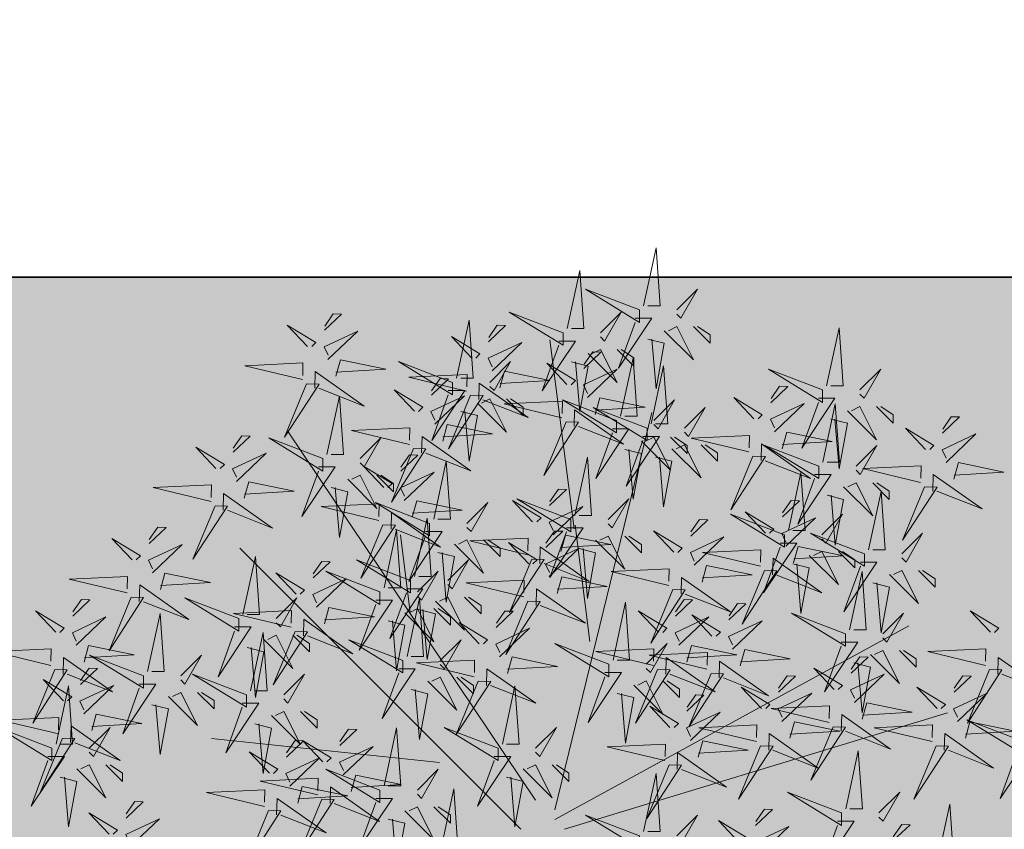
# Model space of a CAD drawing. Units: inches. Extents: x 1704 to 6393, y -157 to 1172.
# Tile 113 of 122: x 2688 to 2716, y 1018 to 1041. Entities that reach past the tile are written whole.
import ezdxf

# ---------------------------------------------------------------- set-up
doc = ezdxf.new("R2010")
doc.units = ezdxf.units.IN
doc.header["$MEASUREMENT"] = 0
for name, color, linetype, lineweight in [('A-ANNO-DIMS', 7, 'Continuous', 13), ('C-PROP', 7, 'Continuous', 35), ('L-shrub', 74, 'Continuous', 18)]:
    doc.layers.add(name, color=color, linetype=linetype, lineweight=lineweight)
doc.layers.add('L-HRDS-PATT', color=9, linetype='Continuous', lineweight=13, true_color=0xc5c1ba)
doc.styles.get("Standard").update_dxf_attribs({"font": 'arial.ttf'})
doc.dimstyles.get("Standard").update_dxf_attribs({"dimtxt": 6, "dimasz": 2, "dimexe": 0.18, "dimexo": 0.0625, "dimgap": 0.09, "dimtad": 0, "dimtih": 1, "dimtoh": 1, "dimdec": 1, "dimzin": 0, "dimdsep": 46, "dimlunit": 3, "dimtxsty": 'Standard', "dimblk": 'ARCHTICK', "dimcen": 0.09, "dimadec": 0, "dimazin": 0, "dimtfac": 1, "dimtdec": 1, "dimtofl": 0, "dimtmove": 0, "dimatfit": 3, "dimfxl": 1, "dimtolj": 1, "dimtzin": 0, "dimarcsym": 0})

# ---------------------------------------------------------------- blocks, each defined once
blk = doc.blocks.new('shrub3')
for p, q in [((-11.38, -5.19), (-224.23, -69.78)), ((12.87, -5.19), (169.14, -161.27)), ((-5.99, -10.57), (-202.68, -118.21)), ((-5.99, -15.96), (-59.88, -236.62)), ((4.78, -21.34), (142.19, -225.85)), ((58.17, -42.16), (184.8, -55.61)), ((-17.27, -174.02), (-25.36, -109.43)), ((74.33, -125.58), (79.72, -168.64)), ((-16.77, -172.03), (-3.3, -276.98))]:
    blk.add_line(p, q)
for points in [[(-163.04, -9.56), (-172.27, -9.56), (-153.8, 18.11), (-163.04, -7.25)], [(86.56, -10.73), (77.32, -8.43), (81.94, 16.94), (84.25, -10.73)], [(-218.53, 13.17), (-225.46, -19.11), (-227.77, 13.17), (-220.84, 13.17)], [(153.14, -15.45), (165.42, 14.26), (146.23, -15.28), (153.14, -15.45)], [(-119.49, 9.1), (-136.03, -6.65), (-117.36, 2.12), (-119.55, 6.79)], [(123.46, -21.81), (135.74, 7.91), (116.55, -21.63), (123.46, -21.81)], [(-193.91, 1.36), (-203.36, -7.64), (-198.75, -7.76), (-193.97, -0.95)], [(-108.14, 1.89), (-96.9, -9.94), (-112.81, -0.3), (-110.44, 1.95)], [(-73.76, -1.46), (-85.3, -12.99), (-76.07, 3.15), (-73.76, 0.84)], [(-52.98, -1.46), (-22.97, -12.99), (-52.98, 5.45), (-52.98, -1.46)], [(57.07, 4.7), (50.14, -27.58), (47.83, 4.7), (54.76, 4.7)], [(77.32, -15.34), (61.16, 0.8), (70.4, -17.65), (75.02, -15.34)], [(93.49, -22.26), (84.25, -22.26), (102.72, 5.41), (93.49, -19.96)], [(230.31, 4.87), (213.77, -10.89), (232.44, -2.12), (230.25, 2.56)], [(-55.29, -3.77), (-62.22, -36.05), (-64.53, -3.77), (-57.6, -3.77)], [(148.59, -13.03), (148.36, -22.26), (121.16, -3.11), (146.29, -12.97)], [(241.66, -2.35), (252.9, -14.18), (237, -4.54), (239.36, -2.29)], [(-186.12, -14.17), (-197.67, -25.7), (-188.43, -9.56), (-186.12, -11.86)], [(-165.34, -14.17), (-135.33, -25.7), (-165.34, -7.25), (-165.34, -14.17)], [(-117.59, -7.11), (-127.04, -16.11), (-122.43, -16.23), (-117.65, -9.42)], [(20.84, -34.02), (11.6, -31.72), (16.22, -6.36), (18.53, -34.02)], [(61.16, -17.65), (51.93, -8.43), (51.93, -13.04), (58.86, -17.65)], [(118.91, -19.38), (118.68, -28.61), (91.48, -9.46), (116.61, -19.33)], [(268.88, -34.02), (259.65, -31.72), (264.26, -6.36), (266.57, -34.02)], [(-69.46, -40.86), (-57.18, -11.15), (-76.37, -40.69), (-69.46, -40.86)], [(232.21, -11.35), (222.76, -20.35), (227.37, -20.46), (232.16, -13.66)], [(-217.86, -51.45), (-205.58, -21.74), (-224.77, -51.28), (-217.86, -51.45)], [(-167.65, -16.47), (-174.58, -48.76), (-176.89, -16.47), (-169.96, -16.47)], [(-120.34, -51.45), (-108.06, -21.74), (-127.25, -51.28), (-120.34, -51.45)], [(27.76, -45.55), (18.53, -45.55), (37, -17.88), (27.76, -43.25)], [(91.18, -26.87), (121.19, -38.4), (91.18, -19.96), (91.18, -26.87)], [(136.89, -19.67), (134.36, -28.84), (109.12, -23.59), (136.84, -21.97)], [(155.39, -17.82), (187.49, -25.55), (155.16, -27.05), (155.33, -20.13)], [(275.81, -45.55), (266.57, -45.55), (285.04, -17.88), (275.81, -43.25)], [(-262.68, -49.79), (-271.91, -49.79), (-253.44, -22.12), (-262.68, -47.48)], [(11.6, -38.64), (-4.56, -22.5), (4.68, -40.94), (9.3, -38.64)], [(70.4, -26.87), (58.86, -38.4), (68.09, -22.26), (70.4, -24.57)], [(107.21, -26.02), (104.68, -35.19), (79.44, -29.94), (107.16, -28.33)], [(125.71, -24.17), (157.81, -31.9), (125.48, -33.4), (125.65, -26.48)], [(259.65, -38.64), (243.49, -22.5), (252.72, -40.94), (257.34, -38.64)], [(267.62, -55.68), (279.9, -25.97), (260.71, -55.51), (267.62, -55.68)], [(-160.62, -62.04), (-148.34, -32.32), (-167.53, -61.86), (-160.62, -62.04)], [(-74.01, -38.44), (-74.24, -47.67), (-101.44, -28.52), (-76.31, -38.38)], [(-4.56, -40.94), (-13.79, -31.72), (-13.79, -36.33), (-6.86, -40.94)], [(88.87, -29.18), (81.94, -61.46), (79.63, -29.18), (86.56, -29.18)], [(141.27, -29.01), (124.73, -44.76), (143.4, -35.99), (141.21, -31.32)], [(243.49, -40.94), (234.25, -31.72), (234.25, -36.33), (241.18, -40.94)], [(111.59, -35.37), (95.05, -51.12), (113.72, -42.35), (111.53, -37.67)], [(152.62, -36.23), (163.86, -48.05), (147.96, -38.42), (150.32, -36.17)], [(160.76, -63.67), (151.53, -61.36), (156.14, -36), (158.45, -63.67)], [(-222.41, -49.03), (-222.64, -58.26), (-249.84, -39.1), (-224.72, -48.97)], [(-124.89, -49.03), (-125.12, -58.26), (-152.32, -39.1), (-127.2, -48.97)], [(-67.21, -43.23), (-35.11, -50.96), (-67.44, -52.46), (-67.27, -45.54)], [(25.46, -50.16), (55.47, -61.69), (25.46, -43.25), (25.46, -50.16)], [(122.94, -42.58), (134.18, -54.41), (118.28, -44.77), (120.64, -42.52)], [(263.07, -53.26), (262.84, -62.49), (235.64, -43.34), (260.77, -53.2)], [(273.5, -50.16), (303.51, -61.69), (273.5, -43.25), (273.5, -50.16)], [(-264.99, -54.4), (-234.97, -65.93), (-264.99, -47.48), (-264.99, -54.4)], [(-85.71, -45.07), (-88.24, -54.25), (-113.48, -49), (-85.77, -47.38)], [(4.68, -50.16), (-6.86, -61.69), (2.37, -45.55), (4.68, -47.86)], [(143.17, -45.23), (133.72, -54.23), (138.33, -54.34), (143.12, -47.53)], [(167.69, -75.2), (158.45, -75.2), (176.92, -47.53), (167.69, -72.89)], [(218, -74.25), (208.77, -71.95), (213.38, -46.59), (215.69, -74.25)], [(252.72, -50.16), (241.18, -61.69), (250.41, -45.55), (252.72, -47.86)], [(-215.61, -53.82), (-183.51, -61.55), (-215.84, -63.05), (-215.67, -56.12)], [(-165.17, -59.61), (-165.4, -68.85), (-192.6, -49.69), (-167.48, -59.56)], [(-118.09, -53.82), (-85.99, -61.55), (-118.32, -63.05), (-118.15, -56.12)], [(-81.33, -54.42), (-97.87, -70.17), (-79.2, -61.4), (-81.39, -56.73)], [(-40.64, -80.61), (-49.88, -78.3), (-45.26, -52.94), (-42.95, -80.61)], [(23.15, -52.47), (16.22, -84.75), (13.91, -52.47), (20.84, -52.47)], [(113.49, -51.58), (104.04, -60.58), (108.65, -60.69), (113.43, -53.89)], [(151.53, -68.28), (135.37, -52.14), (144.6, -70.59), (149.22, -68.28)], [(271.19, -52.47), (264.26, -84.75), (261.95, -52.47), (268.88, -52.47)], [(-234.11, -55.66), (-236.65, -64.84), (-261.89, -59.59), (-234.17, -57.97)], [(-136.59, -55.66), (-139.12, -64.84), (-164.36, -59.59), (-136.65, -57.97)], [(36.54, -87.45), (48.82, -57.73), (29.63, -87.27), (36.54, -87.45)], [(73.84, -82.72), (64.6, -80.42), (69.22, -55.06), (71.53, -82.72)], [(224.93, -85.78), (215.69, -85.78), (234.16, -58.11), (224.93, -83.48)], [(251.37, -59.9), (248.84, -69.07), (223.6, -63.82), (251.32, -62.2)], [(269.87, -58.05), (301.97, -65.78), (269.64, -67.28), (269.81, -60.36)], [(-247.54, -93.8), (-235.26, -64.08), (-254.45, -93.62), (-247.54, -93.8)], [(-229.73, -65.01), (-246.27, -80.76), (-227.6, -71.99), (-229.79, -67.32)], [(-158.37, -64.4), (-126.27, -72.13), (-158.6, -73.63), (-158.43, -66.71)], [(-132.21, -65.01), (-148.75, -80.76), (-130.08, -71.99), (-132.27, -67.32)], [(-92.78, -91.68), (-80.5, -61.97), (-99.69, -91.51), (-92.78, -91.68)], [(-69.98, -61.63), (-58.74, -73.46), (-74.65, -63.83), (-72.28, -61.58)], [(-63.1, -93.8), (-50.82, -64.08), (-70.01, -93.62), (-63.1, -93.8)], [(-33.72, -92.14), (-42.95, -92.14), (-24.48, -64.47), (-33.72, -89.83)], [(135.37, -70.59), (126.13, -61.36), (126.13, -65.97), (133.06, -70.59)], [(208.77, -78.87), (192.61, -62.73), (201.84, -81.17), (206.46, -78.87)], [(271.86, -93.8), (284.14, -64.08), (264.95, -93.62), (271.86, -93.8)], [(-176.87, -66.25), (-179.4, -75.42), (-204.64, -70.17), (-176.93, -68.56)], [(-172.08, -97.55), (-181.32, -95.24), (-176.7, -69.88), (-174.39, -97.55)], [(-79.43, -70.63), (-88.88, -79.64), (-84.27, -79.75), (-79.49, -72.94)], [(-49.88, -85.22), (-66.04, -69.08), (-56.8, -87.52), (-52.18, -85.22)], [(80.77, -94.25), (71.53, -94.25), (90, -66.58), (80.77, -91.95)], [(255.75, -69.24), (239.21, -85), (257.88, -76.23), (255.7, -71.55)], [(-218.38, -72.22), (-207.14, -84.05), (-223.05, -74.41), (-220.68, -72.16)], [(-172.49, -75.6), (-189.03, -91.35), (-170.36, -82.58), (-172.55, -77.9)], [(-120.86, -72.22), (-109.62, -84.05), (-125.53, -74.41), (-123.16, -72.16)], [(31.99, -85.02), (31.76, -94.25), (4.56, -75.1), (29.69, -84.96)], [(64.6, -87.34), (48.44, -71.2), (57.68, -89.64), (62.3, -87.34)], [(144.6, -79.81), (133.06, -91.34), (142.29, -75.2), (144.6, -77.5)], [(165.38, -79.81), (195.39, -91.34), (165.38, -72.89), (165.38, -79.81)], [(192.61, -81.17), (183.37, -71.95), (183.37, -76.56), (190.3, -81.17)], [(267.1, -76.46), (278.34, -88.28), (262.44, -78.65), (264.8, -76.4)], [(-252.09, -91.37), (-252.32, -100.61), (-279.52, -81.45), (-254.4, -91.32)], [(-227.83, -81.22), (-237.28, -90.22), (-232.67, -90.34), (-227.89, -83.53)], [(-165.16, -109.08), (-174.39, -109.08), (-155.92, -81.41), (-165.16, -106.77)], [(-130.31, -81.22), (-139.76, -90.22), (-135.15, -90.34), (-130.37, -83.53)], [(-97.33, -89.26), (-97.56, -98.49), (-124.76, -79.33), (-99.63, -89.2)], [(-67.65, -91.37), (-67.88, -100.61), (-95.08, -81.45), (-69.95, -91.32)], [(-66.04, -87.52), (-75.27, -78.3), (-75.27, -82.91), (-68.34, -87.52)], [(48.44, -89.64), (39.21, -80.42), (39.21, -85.03), (46.14, -89.64)], [(165, -106.02), (155.77, -103.71), (160.38, -78.35), (162.69, -106.02)], [(267.31, -91.37), (267.08, -100.61), (239.88, -81.45), (265.01, -91.32)], [(-181.32, -102.16), (-197.48, -86.02), (-188.24, -104.46), (-183.63, -102.16)], [(-161.14, -82.81), (-149.9, -94.64), (-165.81, -85), (-163.44, -82.75)], [(138.3, -114.97), (150.58, -85.26), (131.39, -114.8), (138.3, -114.97)], [(163.07, -82.11), (156.14, -114.39), (153.83, -82.11), (160.76, -82.11)], [(201.84, -90.4), (190.3, -101.92), (199.53, -85.78), (201.84, -88.09)], [(222.62, -90.4), (252.63, -101.92), (222.62, -83.48), (222.62, -90.4)], [(257.65, -85.46), (248.2, -94.46), (252.81, -94.57), (257.6, -87.76)], [(-170.59, -91.81), (-180.04, -100.81), (-175.43, -100.93), (-170.65, -94.12)], [(-56.8, -96.75), (-68.34, -108.28), (-59.11, -92.14), (-56.8, -94.44)], [(-36.02, -96.75), (-6.01, -108.28), (-36.02, -89.83), (-36.02, -96.75)], [(20.29, -91.66), (17.76, -100.83), (-7.48, -95.58), (20.23, -93.97)], [(38.79, -89.81), (70.89, -97.54), (38.56, -99.04), (38.73, -92.12)], [(78.46, -98.86), (108.47, -110.39), (78.46, -91.95), (78.46, -98.86)], [(171.93, -117.54), (162.69, -117.54), (181.16, -89.88), (171.93, -115.24)], [(220.31, -92.7), (213.38, -124.98), (211.07, -92.7), (218, -92.7)], [(-245.29, -96.16), (-213.19, -103.89), (-245.52, -105.4), (-245.35, -98.47)], [(-197.48, -104.46), (-206.71, -95.24), (-206.71, -99.85), (-199.79, -104.46)], [(-109.03, -95.89), (-111.56, -105.07), (-136.8, -99.82), (-109.09, -98.2)], [(-79.35, -98.01), (-81.88, -107.18), (-107.12, -101.93), (-79.41, -100.32)], [(-90.53, -94.05), (-58.43, -101.78), (-90.76, -103.28), (-90.59, -96.35)], [(-60.85, -96.16), (-28.75, -103.89), (-61.08, -105.4), (-60.91, -98.47)], [(57.68, -98.86), (46.14, -110.39), (55.37, -94.25), (57.68, -96.56)], [(86.56, -120.84), (77.32, -118.53), (81.94, -93.17), (84.25, -120.84)], [(155.77, -110.63), (139.61, -94.49), (148.84, -112.93), (153.46, -110.63)], [(255.61, -98.01), (253.08, -107.18), (227.84, -101.93), (255.56, -100.32)], [(274.11, -96.16), (306.21, -103.89), (273.88, -105.4), (274.05, -98.47)], [(-38.33, -99.05), (-45.26, -131.33), (-47.57, -99.05), (-40.64, -99.05)], [(8.98, -131.91), (21.26, -102.2), (2.07, -131.74), (8.98, -131.91)], [(24.67, -101), (8.13, -116.76), (26.8, -107.99), (24.61, -103.31)], [(69.6, -127.19), (60.36, -124.88), (64.98, -99.52), (67.29, -127.19)], [(76.15, -101.17), (69.22, -133.45), (66.91, -101.17), (73.84, -101.17)], [(133.75, -112.55), (133.52, -121.78), (106.32, -102.62), (131.45, -112.49)], [(139.61, -112.93), (130.37, -103.71), (130.37, -108.32), (137.3, -112.93)], [(-188.24, -113.69), (-199.79, -125.22), (-190.55, -109.08), (-188.24, -111.38)], [(-167.46, -113.69), (-137.45, -125.22), (-167.46, -106.77), (-167.46, -113.69)], [(-104.65, -105.24), (-121.19, -120.99), (-102.52, -112.22), (-104.71, -107.55)], [(-74.97, -107.36), (-91.51, -123.11), (-72.84, -114.34), (-75.03, -109.66)], [(-71.58, -138.26), (-59.3, -108.55), (-78.49, -138.09), (-71.58, -138.26)], [(36.02, -108.22), (47.26, -120.04), (31.36, -110.41), (33.72, -108.16)], [(77.32, -125.45), (61.16, -109.31), (70.4, -127.75), (75.02, -125.45)], [(93.49, -132.37), (84.25, -132.37), (102.72, -104.7), (93.49, -130.06)], [(229.46, -134.03), (241.74, -104.31), (222.55, -133.86), (229.46, -134.03)], [(259.99, -107.36), (243.45, -123.11), (262.12, -114.34), (259.94, -109.66)], [(-248.06, -114.57), (-236.82, -126.4), (-252.73, -116.76), (-250.36, -114.51)], [(-182.68, -142.01), (-191.92, -139.71), (-187.3, -114.34), (-184.99, -142.01)], [(-93.3, -112.45), (-82.06, -124.28), (-97.97, -114.64), (-95.6, -112.39)], [(-63.62, -114.57), (-52.38, -126.4), (-68.29, -116.76), (-65.92, -114.51)], [(76.53, -138.72), (67.29, -138.72), (85.76, -111.05), (76.53, -136.41)], [(271.34, -114.57), (282.58, -126.4), (266.68, -116.76), (269.04, -114.51)], [(-169.77, -115.99), (-176.7, -148.27), (-179.01, -115.99), (-172.08, -115.99)], [(-122.46, -148.85), (-110.18, -119.14), (-129.37, -148.68), (-122.46, -148.85)], [(4.43, -129.49), (4.2, -138.72), (-23, -119.56), (2.13, -129.43)], [(26.57, -117.22), (17.12, -126.22), (21.73, -126.33), (26.51, -119.53)], [(60.36, -131.8), (44.2, -115.66), (53.44, -134.11), (58.06, -131.8)], [(61.16, -127.75), (51.93, -118.53), (51.93, -123.14), (58.86, -127.75)], [(122.05, -119.18), (119.52, -128.36), (94.28, -123.11), (122, -121.49)], [(148.84, -122.16), (137.3, -133.69), (146.53, -117.54), (148.84, -119.85)], [(140.55, -117.34), (172.65, -125.07), (140.32, -126.57), (140.49, -119.65)], [(169.62, -122.16), (199.63, -133.69), (169.62, -115.24), (169.62, -122.16)], [(-138.16, -152.6), (-147.4, -150.29), (-142.78, -124.93), (-140.47, -152.6)], [(-102.75, -121.45), (-112.2, -130.45), (-107.59, -130.57), (-102.81, -123.76)], [(-73.07, -123.57), (-82.52, -132.57), (-77.91, -132.69), (-73.13, -125.88)], [(6.86, -155.2), (19.14, -125.49), (-0.05, -155.03), (6.86, -155.2)], [(44.2, -134.11), (34.97, -124.88), (34.97, -129.5), (41.9, -134.11)], [(167.31, -124.46), (160.38, -156.74), (158.07, -124.46), (165, -124.46)], [(224.91, -131.61), (224.68, -140.84), (197.48, -121.68), (222.61, -131.55)], [(261.89, -123.57), (252.44, -132.57), (257.05, -132.69), (261.84, -125.88)], [(-191.92, -146.62), (-208.08, -130.48), (-198.84, -148.93), (-194.23, -146.62)], [(-175.76, -153.54), (-184.99, -153.54), (-166.52, -125.87), (-175.76, -151.23)], [(-76.13, -135.84), (-76.36, -145.07), (-103.56, -125.92), (-78.43, -135.78)], [(59, -158.95), (49.76, -156.64), (54.38, -131.28), (56.69, -158.95)], [(91.18, -136.98), (121.19, -148.51), (91.18, -130.06), (91.18, -136.98)], [(126.43, -128.53), (109.89, -144.28), (128.56, -135.51), (126.37, -130.84)], [(-127.01, -146.43), (-127.24, -155.66), (-154.44, -136.5), (-129.32, -146.37)], [(-131.24, -164.13), (-140.47, -164.13), (-122, -136.46), (-131.24, -161.82)], [(-7.27, -136.12), (-9.8, -145.3), (-35.04, -140.05), (-7.33, -138.43)], [(-19.44, -161.07), (-28.68, -158.76), (-24.06, -133.4), (-21.75, -161.07)], [(11.23, -134.28), (43.33, -142.01), (11, -143.51), (11.17, -136.58)], [(70.4, -136.98), (58.86, -148.51), (68.09, -132.37), (70.4, -134.67)], [(74.22, -143.33), (104.23, -154.86), (74.22, -136.41), (74.22, -143.33)], [(137.78, -135.74), (149.02, -147.57), (133.12, -137.94), (135.48, -135.69)], [(231.71, -136.39), (263.81, -144.13), (231.48, -145.63), (231.65, -138.7)], [(-208.08, -148.93), (-217.31, -139.71), (-217.31, -144.32), (-210.39, -148.93)], [(-147.4, -157.21), (-163.56, -141.07), (-154.32, -159.52), (-149.71, -157.21)], [(-69.33, -140.63), (-37.23, -148.36), (-69.56, -149.86), (-69.39, -142.94)], [(53.44, -143.33), (41.9, -154.86), (51.13, -138.72), (53.44, -141.02)], [(88.87, -139.28), (81.94, -171.56), (79.63, -139.28), (86.56, -139.28)], [(213.21, -138.24), (210.68, -147.41), (185.44, -142.16), (213.16, -140.55)], [(-87.83, -142.48), (-90.36, -151.65), (-115.6, -146.4), (-87.89, -144.78)], [(2.31, -152.78), (2.08, -162.01), (-25.12, -142.86), (0.01, -152.72)], [(-12.52, -172.6), (-21.75, -172.6), (-3.28, -144.93), (-12.52, -170.29)], [(-2.89, -145.47), (-19.43, -161.22), (-0.76, -152.45), (-2.95, -147.78)], [(49.76, -163.56), (33.6, -147.42), (42.84, -165.87), (47.46, -163.56)], [(65.93, -170.48), (56.69, -170.48), (75.16, -142.81), (65.93, -168.17)], [(71.91, -145.64), (64.98, -177.92), (62.67, -145.64), (69.6, -145.64)], [(89.54, -174.26), (101.82, -144.54), (82.63, -174.09), (89.54, -174.26)], [(128.33, -144.74), (118.88, -153.74), (123.49, -153.86), (128.27, -147.05)], [(217.59, -147.59), (201.05, -163.34), (219.72, -154.57), (217.53, -149.9)], [(-178.06, -158.15), (-148.05, -169.68), (-178.06, -151.23), (-178.06, -158.15)], [(-163.56, -159.52), (-172.79, -150.29), (-172.79, -154.9), (-165.87, -159.52)], [(-138.71, -153.06), (-141.24, -162.24), (-166.48, -156.99), (-138.77, -155.37)], [(-120.21, -151.22), (-88.11, -158.95), (-120.44, -160.45), (-120.27, -153.52)], [(-83.45, -151.82), (-99.99, -167.57), (-81.32, -158.8), (-83.51, -154.13)], [(-28.68, -165.68), (-44.84, -149.54), (-35.6, -167.99), (-30.98, -165.68)], [(8.46, -152.68), (19.7, -164.51), (3.8, -154.87), (6.16, -152.62)], [(-198.84, -158.15), (-210.39, -169.68), (-201.15, -153.54), (-198.84, -155.85)], [(9.11, -157.57), (41.21, -165.3), (8.88, -166.8), (9.05, -159.88)], [(33.6, -165.87), (24.37, -156.64), (24.37, -161.26), (31.3, -165.87)], [(182.82, -184.85), (195.1, -155.13), (175.91, -184.67), (182.82, -184.85)], [(228.94, -154.8), (240.18, -166.63), (224.28, -156.99), (226.64, -154.74)], [(-180.37, -160.46), (-187.3, -192.74), (-189.61, -160.46), (-182.68, -160.46)], [(-157.24, -190.71), (-166.48, -188.41), (-161.86, -163.04), (-159.55, -190.71)], [(-154.32, -168.74), (-165.87, -180.27), (-156.63, -164.13), (-154.32, -166.43)], [(-134.33, -162.41), (-150.87, -178.16), (-132.2, -169.39), (-134.39, -164.72)], [(-133.54, -168.74), (-103.53, -180.27), (-133.54, -161.82), (-133.54, -168.74)], [(-72.1, -159.03), (-60.86, -170.86), (-76.77, -161.23), (-74.4, -158.98)], [(-44.84, -167.99), (-54.07, -158.76), (-54.07, -163.37), (-47.14, -167.99)], [(-9.39, -159.41), (-11.92, -168.59), (-37.16, -163.34), (-9.45, -161.72)], [(-0.99, -161.68), (-10.44, -170.68), (-5.83, -170.8), (-1.05, -163.99)], [(84.99, -171.84), (84.76, -181.07), (57.56, -161.91), (82.69, -171.78)], [(219.49, -163.8), (210.04, -172.8), (214.65, -172.92), (219.44, -166.11)], [(-211.5, -195.43), (-199.22, -165.72), (-218.41, -195.26), (-211.5, -195.43)], [(-122.98, -169.62), (-111.74, -181.45), (-127.65, -171.81), (-125.28, -169.56)], [(-81.55, -168.04), (-91, -177.04), (-86.39, -177.15), (-81.61, -170.34)], [(-5.01, -168.76), (-21.55, -184.51), (-2.88, -175.74), (-5.07, -171.07)], [(63.62, -175.09), (93.63, -186.62), (63.62, -168.17), (63.62, -175.09)], [(118.36, -194.95), (109.13, -192.64), (113.74, -167.28), (116.05, -194.95)], [(-150.32, -202.24), (-159.55, -202.24), (-141.08, -174.57), (-150.32, -199.93)], [(-135.85, -171.04), (-142.78, -203.33), (-145.09, -171.04), (-138.16, -171.04)], [(-35.6, -177.21), (-47.14, -188.74), (-37.91, -172.6), (-35.6, -174.9)], [(-14.82, -177.21), (15.19, -188.74), (-14.82, -170.29), (-14.82, -177.21)], [(42.84, -175.09), (31.3, -186.62), (40.53, -170.48), (42.84, -172.79)], [(178.27, -182.42), (178.04, -191.65), (150.84, -172.5), (175.97, -182.36)], [(-166.48, -195.32), (-182.64, -179.18), (-173.4, -197.63), (-168.79, -195.32)], [(-132.43, -178.62), (-141.88, -187.62), (-137.27, -187.74), (-132.49, -180.93)], [(-17.13, -179.51), (-24.06, -211.79), (-26.37, -179.51), (-19.44, -179.51)], [(6.34, -175.97), (17.58, -187.8), (1.68, -178.17), (4.04, -175.92)], [(73.29, -178.47), (70.76, -187.64), (45.52, -182.39), (73.23, -180.78)], [(61.31, -177.4), (54.38, -209.68), (52.07, -177.4), (59, -177.4)], [(91.79, -176.62), (123.89, -184.36), (91.56, -185.86), (91.73, -178.93)], [(125.29, -206.48), (116.05, -206.48), (134.52, -178.81), (125.29, -204.17)], [(-216.05, -193.01), (-216.28, -202.24), (-243.48, -183.09), (-218.36, -192.95)], [(-116.1, -212.37), (-103.82, -182.66), (-123.01, -212.2), (-116.1, -212.37)], [(-61.84, -211.89), (-71.08, -209.58), (-66.46, -184.22), (-64.15, -211.89)], [(-3.11, -184.97), (-12.56, -193.97), (-7.95, -194.09), (-3.17, -187.28)], [(109.13, -199.56), (92.96, -183.42), (102.2, -201.86), (106.82, -199.56)], [(-182.64, -197.63), (-191.87, -188.41), (-191.87, -193.02), (-184.95, -197.63)], [(-44.88, -216.12), (-54.12, -213.81), (-49.5, -188.45), (-47.19, -216.12)], [(77.67, -187.82), (61.13, -203.57), (79.8, -194.8), (77.61, -190.13)], [(72.58, -216.61), (84.86, -186.89), (65.67, -216.43), (72.58, -216.61)], [(166.57, -189.06), (164.04, -198.23), (138.8, -192.98), (166.52, -191.37)], [(185.07, -187.21), (217.17, -194.94), (184.84, -196.44), (185.01, -189.52)], [(-54.92, -223.41), (-64.15, -223.41), (-45.68, -195.75), (-54.92, -221.11)], [(92.96, -201.86), (83.73, -192.64), (83.73, -197.25), (90.66, -201.86)], [(89.02, -195.03), (100.26, -206.86), (84.36, -197.22), (86.72, -194.97)], [(-227.75, -199.64), (-230.29, -208.82), (-255.53, -203.57), (-227.81, -201.95)], [(-209.25, -197.8), (-177.15, -205.53), (-209.48, -207.03), (-209.31, -200.11)], [(-173.4, -206.85), (-184.95, -218.38), (-175.71, -202.24), (-173.4, -204.55)], [(-152.62, -206.85), (-122.61, -218.38), (-152.62, -199.93), (-152.62, -206.85)], [(-120.65, -209.95), (-120.88, -219.18), (-148.08, -200.02), (-122.96, -209.89)], [(-71.08, -216.5), (-87.24, -200.36), (-78, -218.8), (-73.38, -216.5)], [(-37.96, -227.65), (-47.19, -227.65), (-28.72, -199.98), (-37.96, -225.34)], [(-12.22, -231.43), (0.06, -201.71), (-19.13, -231.26), (-12.22, -231.43)], [(170.95, -198.4), (154.41, -214.16), (173.08, -205.39), (170.89, -200.71)], [(-159.36, -233.06), (-168.6, -230.75), (-163.98, -205.39), (-161.67, -233.06)], [(-54.12, -220.73), (-70.28, -204.59), (-61.04, -223.04), (-56.42, -220.73)], [(68.03, -214.18), (67.8, -223.42), (40.6, -204.26), (65.73, -214.13)], [(79.57, -204.03), (70.12, -213.03), (74.73, -213.15), (79.51, -206.34)], [(102.2, -211.09), (90.66, -222.62), (99.89, -206.48), (102.2, -208.78)], [(122.98, -211.09), (152.99, -222.62), (122.98, -204.17), (122.98, -211.09)], [(182.3, -205.62), (193.54, -217.44), (177.64, -207.81), (180, -205.56)], [(-223.37, -208.99), (-239.91, -224.74), (-221.24, -215.97), (-223.43, -211.3)], [(-154.93, -209.16), (-161.86, -241.44), (-164.17, -209.16), (-157.24, -209.16)], [(-87.24, -218.8), (-96.47, -209.58), (-96.47, -214.19), (-89.54, -218.8)], [(46.28, -237.29), (37.04, -234.99), (41.66, -209.63), (43.97, -237.29)], [(-212.02, -216.2), (-200.78, -228.03), (-216.69, -218.4), (-214.32, -216.15)], [(-152.44, -244.59), (-161.67, -244.59), (-143.2, -216.92), (-152.44, -242.28)], [(-132.35, -216.58), (-134.88, -225.76), (-160.12, -220.51), (-132.41, -218.89)], [(-113.85, -214.74), (-81.75, -222.47), (-114.08, -223.97), (-113.91, -217.05)], [(-70.28, -223.04), (-79.51, -213.81), (-79.51, -218.43), (-72.58, -223.04)], [(40.78, -246.25), (53.06, -216.54), (33.87, -246.08), (40.78, -246.25)], [(120.67, -213.39), (113.74, -245.67), (111.43, -213.39), (118.36, -213.39)], [(172.85, -214.62), (163.4, -223.62), (168.01, -223.73), (172.8, -216.93)], [(-168.6, -237.67), (-184.76, -221.53), (-175.52, -239.98), (-170.91, -237.67)], [(-78, -228.03), (-89.54, -239.55), (-80.31, -223.41), (-78, -225.72)], [(-57.22, -228.03), (-27.21, -239.55), (-57.22, -221.11), (-57.22, -228.03)], [(-16.77, -229.01), (-17, -238.24), (-44.2, -219.08), (-19.07, -228.95)], [(56.33, -220.82), (53.8, -229.99), (28.56, -224.74), (56.27, -223.13)], [(53.21, -248.82), (43.97, -248.82), (62.44, -221.15), (53.21, -246.52)], [(74.83, -218.97), (106.93, -226.7), (74.6, -228.2), (74.77, -221.28)], [(131.94, -252.6), (144.22, -222.89), (125.03, -252.43), (131.94, -252.6)], [(-221.47, -225.2), (-230.92, -234.21), (-226.31, -234.32), (-221.53, -227.51)], [(-127.97, -225.93), (-144.51, -241.68), (-125.84, -232.91), (-128.03, -228.24)], [(-61.04, -232.26), (-72.58, -243.79), (-63.35, -227.65), (-61.04, -229.95)], [(-40.26, -232.26), (-10.25, -243.79), (-40.26, -225.34), (-40.26, -232.26)], [(37.04, -241.91), (20.88, -225.77), (30.12, -244.21), (34.74, -241.91)], [(-184.76, -239.98), (-193.99, -230.75), (-193.99, -235.37), (-187.07, -239.98)], [(-116.62, -233.14), (-105.38, -244.97), (-121.29, -235.34), (-118.92, -233.09)], [(-59.53, -230.33), (-66.46, -262.61), (-68.77, -230.33), (-61.84, -230.33)], [(-42.57, -234.57), (-49.5, -266.85), (-51.81, -234.57), (-44.88, -234.57)], [(-9.97, -233.79), (22.13, -241.53), (-10.2, -243.03), (-10.03, -236.1)], [(36.23, -243.83), (36, -253.06), (8.8, -233.9), (33.93, -243.77)], [(20.88, -244.21), (11.65, -234.99), (11.65, -239.6), (18.58, -244.21)], [(60.71, -230.17), (44.17, -245.92), (62.84, -237.15), (60.65, -232.47)], [(-28.47, -235.64), (-31, -244.81), (-56.24, -239.56), (-28.53, -237.95)], [(-15.2, -264.82), (-24.44, -262.51), (-19.82, -237.15), (-17.51, -264.82)], [(72.06, -237.38), (83.3, -249.21), (67.4, -239.57), (69.76, -237.32)], [(127.39, -250.18), (127.16, -259.41), (99.96, -240.26), (125.09, -250.12)], [(-175.52, -249.2), (-187.07, -260.73), (-177.83, -244.59), (-175.52, -246.89)], [(-154.74, -249.2), (-124.73, -260.73), (-154.74, -242.28), (-154.74, -249.2)], [(-126.07, -242.14), (-135.52, -251.14), (-130.91, -251.26), (-126.13, -244.45)], [(-24.09, -244.99), (-40.63, -260.74), (-21.96, -251.97), (-24.15, -247.3)], [(-157.05, -251.51), (-163.98, -283.79), (-166.29, -251.51), (-159.36, -251.51)], [(-57.6, -277.52), (-66.84, -275.22), (-62.22, -249.86), (-59.91, -277.52)], [(-8.28, -276.35), (-17.51, -276.35), (0.96, -248.68), (-8.28, -274.04)], [(24.53, -250.46), (22, -259.64), (-3.24, -254.39), (24.47, -252.77)], [(30.12, -253.43), (18.58, -264.96), (27.81, -248.82), (30.12, -251.13)], [(43.03, -248.62), (75.13, -256.35), (42.8, -257.85), (42.97, -250.92)], [(50.9, -253.43), (80.91, -264.96), (50.9, -246.52), (50.9, -253.43)], [(62.61, -246.38), (53.16, -255.38), (57.77, -255.49), (62.55, -248.69)], [(-24.44, -269.43), (-40.6, -253.29), (-31.36, -271.74), (-26.74, -269.43)], [(-12.74, -252.2), (-1.5, -264.03), (-17.4, -254.39), (-15.04, -252.14)], [(48.59, -255.74), (41.66, -288.02), (39.35, -255.74), (46.28, -255.74)], [(115.69, -256.81), (113.16, -265.99), (87.92, -260.74), (115.64, -259.12)], [(134.19, -254.97), (166.29, -262.7), (133.96, -264.2), (134.13, -257.28)], [(-50.68, -289.05), (-59.91, -289.05), (-41.44, -261.38), (-50.68, -286.75)], [(-40.6, -271.74), (-49.83, -262.51), (-49.83, -267.13), (-42.9, -271.74)], [(-22.19, -261.2), (-31.64, -270.2), (-27.03, -270.32), (-22.25, -263.51)], [(28.91, -259.81), (12.37, -275.56), (31.04, -266.79), (28.85, -262.12)], [(-66.84, -282.14), (-83, -266), (-73.76, -284.44), (-69.14, -282.14)], [(40.26, -267.02), (51.5, -278.85), (35.6, -269.21), (37.96, -266.96)], [(120.07, -266.16), (103.53, -281.91), (122.2, -273.14), (120.01, -268.47)], [(131.42, -273.37), (142.66, -285.2), (126.76, -275.57), (129.12, -273.32)], [(-83, -284.44), (-92.23, -275.22), (-92.23, -279.83), (-85.3, -284.44)], [(-31.36, -280.96), (-42.9, -292.49), (-33.67, -276.35), (-31.36, -278.65)], [(-10.58, -280.96), (19.43, -292.49), (-10.58, -274.04), (-10.58, -280.96)], [(30.81, -276.02), (21.36, -285.02), (25.97, -285.14), (30.75, -278.33)], [(-12.89, -283.27), (-19.82, -315.55), (-22.13, -283.27), (-15.2, -283.27)], [(121.97, -282.37), (112.52, -291.38), (117.13, -291.49), (121.91, -284.68)], [(-73.76, -293.67), (-85.3, -305.19), (-76.07, -289.05), (-73.76, -291.36)], [(-52.98, -293.67), (-22.97, -305.19), (-52.98, -286.75), (-52.98, -293.67)], [(-55.29, -295.97), (-62.22, -328.25), (-64.53, -295.97), (-57.6, -295.97)]]:
    blk.add_lwpolyline(points)
blk = doc.blocks.new('_ArchTick')
at = {"color": 0, "linetype": 'ByBlock', "const_width": 0.15}
blk.add_lwpolyline([(-0.5, -0.5), (0.5, 0.5)], dxfattribs=at)
blk = doc.blocks.new('*D95')
at = {"layer": 'A-ANNO-DIMS', "color": 0, "lineweight": -2, "transparency": 16777216}
for p, q in [((2605.349, 895.275), (2605.349, 1105.287)), ((2723.349, 895.275), (2723.349, 1105.287)), ((2605.349, 1105.107), (2657.907, 1105.107)), ((2723.349, 1105.107), (2670.791, 1105.107))]:
    blk.add_line(p, q, dxfattribs=at)
at = {"layer": 'Defpoints', "color": 0, "lineweight": -3, "transparency": 16777216}
for p in [(2723.349, 1105.107), (2605.349, 895.213), (2723.349, 895.213)]:
    blk.add_point(p, dxfattribs=at)
at = {"layer": 'A-ANNO-DIMS', "color": 0, "lineweight": -2, "transparency": 16777216, "xscale": 2, "yscale": 2, "zscale": 2, "rotation": 180}
blk.add_blockref('_ArchTick', (2605.349, 1105.107), dxfattribs=at)
at = {"layer": 'A-ANNO-DIMS', "color": 0, "lineweight": -2, "transparency": 16777216, "xscale": 2, "yscale": 2, "zscale": 2}
blk.add_blockref('_ArchTick', (2723.349, 1105.107), dxfattribs=at)
at = {"layer": 'A-ANNO-DIMS', "color": 0, "transparency": 16777216, "insert": (2664.349, 1105.107), "char_height": 6, "attachment_point": 5}
blk.add_mtext('\\A1;118', dxfattribs=at)

msp = doc.modelspace()

# ---------------------------------------------------------------- hatches: boundary and pattern name
at = {"layer": 'L-HRDS-PATT', "transparency": 33554661}
h = msp.add_hatch(color=256, dxfattribs=at)
h.dxf.hatch_style = 1
h.paths.add_polyline_path([(2719.349, 1033.213), (2664.349, 1033.213), (2664.349, 895.213), (2719.349, 895.213)])
h.paths.add_polyline_path([(2719.349, 895.213), (2664.349, 895.213), (2605.349, 895.213), (2605.349, 872.213), (2719.349, 872.213)])
h.paths.add_polyline_path([(2719.349, 872.213), (2605.349, 872.213), (2605.349, 854.213), (2601.349, 854.213, -0.121066), (2618.034, 850.113), (2618.05, 850.14), (2619.349, 849.39), (2601.349, 818.213), (2605.349, 818.213), (2605.349, 794.213), (2605.349, 754.213), (2631.349, 754.213), (2631.349, 716.213), (2719.349, 716.213)])

# ---------------------------------------------------------------- linework, layer by layer
at = {"layer": 'C-PROP'}
msp.add_line((2723.349, 1033.213), (1898.349, 1033.213), dxfattribs=at)

# ---------------------------------------------------------------- block references
at = {"layer": 'L-shrub', "xscale": 0.0510581485411622, "yscale": 0.0510581485411622, "zscale": 0.0510581485411622, "rotation": 180}
msp.add_blockref('shrub3', (2703.343, 1017.291), dxfattribs=at)

# ---------------------------------------------------------------- dimensions: what is measured, and where the dimension line sits
at = {"layer": 'A-ANNO-DIMS'}
dim = msp.add_linear_dim(base=(2723.349, 1105.107), p1=(2605.349, 895.213), p2=(2723.349, 895.213), dimstyle='Standard', override={"dimdec": 0, "dimlfac": 1, "dimrnd": 0, "dimzin": 0, "dimdsep": 46, "dimlunit": 2}, dxfattribs=at)
dim.commit()
dim.dimension.update_dxf_attribs({"geometry": '*D95', "text_midpoint": (2664.349, 1105.107)})

doc.saveas('drawing.dxf')
